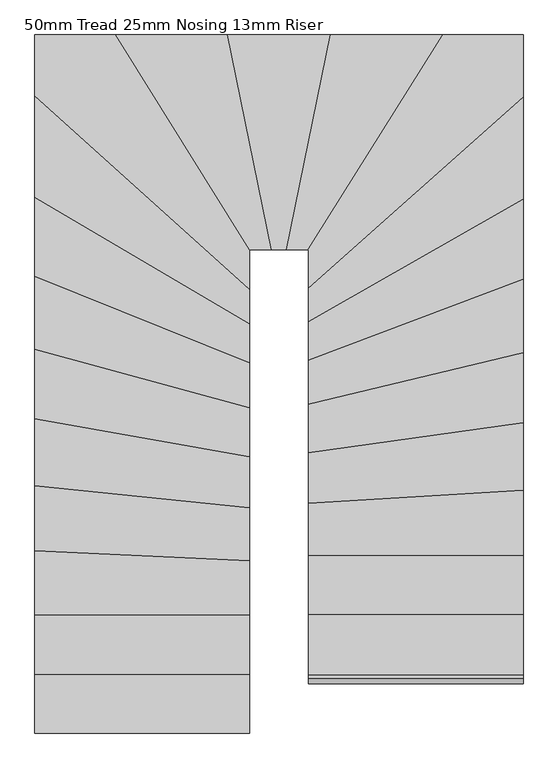
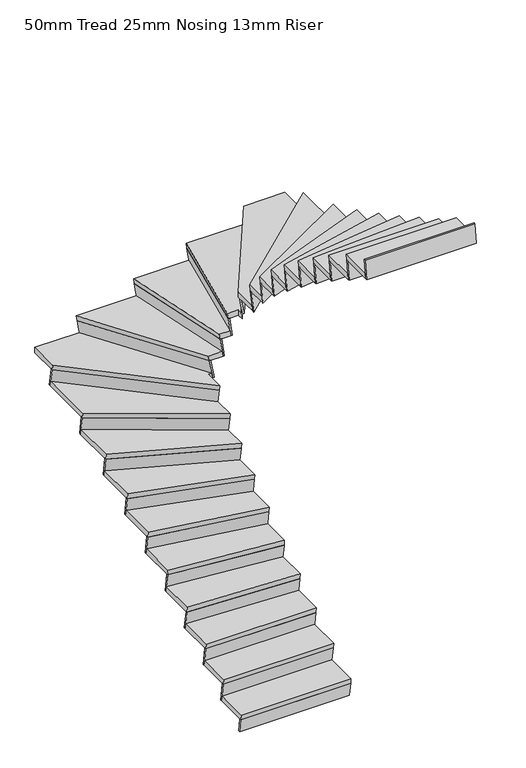
"""IFC4 building model written with IfcOpenShell, lengths in millimetres: stair flight geometry, 50mm Tread 25mm Nosing 13mm Riser."""

from ifc_helpers import new_model, si_unit, origin, place, context, project, spatial, faceted_brep, source, transform, mapped, element, save


def stair_flight_50mm_tread_25mm_nosing_13mm_riser_90fcb94b(model_context):
    return source(origin(), model_context, "Body", "Brep", [
        faceted_brep([(-7658.1394344, -389.3306191, 173.9130435), (-7658.1394344, -382.1431191, 123.9130435), (-8658.1652156, -382.1431191, 123.9130435), (-8658.1652156, -389.3306191, 173.9130435), (-8658.1652156, -689.3306191, 173.9130435), (-7658.1394344, -689.3306191, 173.9130435), (-7658.1394344, -682.1431191, 123.9130435), (-8658.1652156, -682.1431191, 123.9130435)], [[[0, 1, 2, 3]], [[3, 4, 5, 0]], [[2, 1, 6, 7]], [[4, 3, 2, 7]], [[0, 5, 6, 1]], [[5, 4, 7, 6]]]),
        faceted_brep([(-7658.1394344, -682.1431191, 123.9130435), (-7658.1394344, -664.3306191, 0.0), (-7658.1394344, -651.7021291, 0.0), (-7658.1394344, -669.5146291, 123.9130435), (-8658.1652156, -682.1431191, 123.9130435), (-8658.1652156, -669.5146291, 123.9130435), (-8658.1652156, -651.7021291, 0.0), (-8658.1652156, -664.3306191, 0.0)], [[[0, 1, 2, 3]], [[4, 5, 6, 7]], [[1, 0, 4, 7]], [[2, 1, 7, 6]], [[3, 2, 6, 5]], [[0, 3, 5, 4]]]),
        faceted_brep([(-7658.1394344, -407.1431191, 297.826087), (-7658.1394344, -382.1431191, 123.9130435), (-7658.1394344, -369.5146291, 123.9130435), (-7658.1394344, -394.5146291, 297.826087), (-8658.1652156, -407.1431191, 297.826087), (-8658.1652156, -394.5146291, 297.826087), (-8658.1652156, -369.5146291, 123.9130435), (-8658.1652156, -382.1431191, 123.9130435)], [[[0, 1, 2, 3]], [[4, 5, 6, 7]], [[1, 0, 4, 7]], [[2, 1, 7, 6]], [[3, 2, 6, 5]], [[0, 3, 5, 4]]]),
        faceted_brep([(-8658.1652156, -114.3306191, 347.826087), (-8658.1652156, -414.3306191, 347.826087), (-7658.1394344, -414.3306191, 347.826087), (-7658.1394344, -114.3306191, 347.826087), (-8658.1652156, -107.1431191, 297.826087), (-7658.1394344, -107.1431191, 297.826087), (-7658.1394344, -407.1431191, 297.826087), (-8658.1652156, -407.1431191, 297.826087)], [[[0, 1, 2, 3]], [[4, 5, 6, 7]], [[1, 0, 4, 7]], [[3, 2, 6, 5]], [[3, 5, 4, 0]], [[2, 1, 7, 6]]]),
        faceted_brep([(-7658.1394344, -132.1431191, 471.7391304), (-7658.1394344, -107.1431191, 297.826087), (-7658.1394344, -94.5146291, 297.826087), (-7658.1394344, -119.5146291, 471.7391304), (-8658.1652156, -132.1431191, 471.7391304), (-8658.1652156, -119.5146291, 471.7391304), (-8658.1652156, -94.5146291, 297.826087), (-8658.1652156, -107.1431191, 297.826087)], [[[0, 1, 2, 3]], [[4, 5, 6, 7]], [[1, 0, 4, 7]], [[2, 1, 7, 6]], [[3, 2, 6, 5]], [[0, 3, 5, 4]]]),
        faceted_brep([(-8658.1652156, 184.0364565, 521.7391304), (-8658.1652156, -139.3306191, 521.7391304), (-7658.1394344, -139.3306191, 521.7391304), (-7658.1394344, 137.3567478, 521.7391304), (-8658.1652156, 191.2317826, 471.7391304), (-7658.1394344, 144.5520739, 471.7391304), (-7658.1394344, -132.1431191, 471.7391304), (-8658.1652156, -132.1431191, 471.7391304)], [[[0, 1, 2, 3]], [[4, 5, 6, 7]], [[1, 0, 4, 7]], [[3, 2, 6, 5]], [[3, 5, 4, 0]], [[2, 1, 7, 6]]]),
        faceted_brep([(-7658.1394344, 119.5248527, 645.6521739), (-7658.1394344, 144.5520739, 471.7391304), (-7658.1394344, 157.1943144, 471.7391304), (-7658.1394344, 132.1670932, 645.6521739), (-8658.1652156, 166.2045614, 645.6521739), (-8658.1652156, 178.8468019, 645.6521739), (-8658.1652156, 203.8740231, 471.7391304), (-8658.1652156, 191.2317826, 471.7391304)], [[[0, 1, 2, 3]], [[4, 5, 6, 7]], [[1, 0, 4, 7]], [[2, 1, 7, 6]], [[3, 2, 6, 5]], [[0, 3, 5, 4]]]),
        faceted_brep([(-8658.1652156, 487.9562155, 695.6521739), (-8658.1652156, 159.0092353, 695.6521739), (-7658.1394344, 112.3295266, 695.6521739), (-7658.1394344, 383.6537717, 695.6521739), (-8658.1652156, 495.1827041, 645.6521739), (-7658.1394344, 390.8802603, 645.6521739), (-7658.1394344, 119.5248527, 645.6521739), (-8658.1652156, 166.2045614, 645.6521739)], [[[0, 1, 2, 3]], [[4, 5, 6, 7]], [[1, 0, 4, 7]], [[3, 2, 6, 5]], [[3, 5, 4, 0]], [[2, 1, 7, 6]]]),
        faceted_brep([(-7658.1394344, 365.7446477, 819.5652174), (-7658.1394344, 390.8802603, 645.6521739), (-7658.1394344, 403.5772537, 645.6521739), (-7658.1394344, 378.441641, 819.5652174), (-8658.1652156, 470.0470915, 819.5652174), (-8658.1652156, 482.7440848, 819.5652174), (-8658.1652156, 507.8796975, 645.6521739), (-8658.1652156, 495.1827041, 645.6521739)], [[[0, 1, 2, 3]], [[4, 5, 6, 7]], [[1, 0, 4, 7]], [[2, 1, 7, 6]], [[3, 2, 6, 5]], [[0, 3, 5, 4]]]),
        faceted_brep([(-8658.1652156, 799.6725249, 869.5652174), (-8658.1652156, 462.8206028, 869.5652174), (-7658.1394344, 358.518159, 869.5652174), (-7658.1394344, 622.4453627, 869.5652174), (-8658.1652156, 806.9720243, 819.5652174), (-7658.1394344, 629.7448621, 819.5652174), (-7658.1394344, 365.7446477, 819.5652174), (-8658.1652156, 470.0470915, 819.5652174)], [[[0, 1, 2, 3]], [[4, 5, 6, 7]], [[1, 0, 4, 7]], [[3, 2, 6, 5]], [[3, 5, 4, 0]], [[2, 1, 7, 6]]]),
        faceted_brep([(-7658.1394344, 604.3552992, 993.4782609), (-7658.1394344, 629.7448621, 819.5652174), (-7658.1394344, 642.5701357, 819.5652174), (-7658.1394344, 617.1805728, 993.4782609), (-8658.1652156, 781.5824614, 993.4782609), (-8658.1652156, 794.407735, 993.4782609), (-8658.1652156, 819.7972979, 819.5652174), (-8658.1652156, 806.9720243, 819.5652174)], [[[0, 1, 2, 3]], [[4, 5, 6, 7]], [[1, 0, 4, 7]], [[2, 1, 7, 6]], [[3, 2, 6, 5]], [[0, 3, 5, 4]]]),
        faceted_brep([(-8658.1652156, 1122.8219805, 1043.4782609), (-8658.1652156, 774.282962, 1043.4782609), (-7658.1394344, 597.0557998, 1043.4782609), (-7658.1394344, 850.3396239, 1043.4782609), (-8658.1652156, 1130.2715142, 993.4782609), (-7658.1394344, 857.7891576, 993.4782609), (-7658.1394344, 604.3552992, 993.4782609), (-8658.1652156, 781.5824614, 993.4782609)], [[[0, 1, 2, 3]], [[4, 5, 6, 7]], [[1, 0, 4, 7]], [[3, 2, 6, 5]], [[3, 5, 4, 0]], [[2, 1, 7, 6]]]),
        faceted_brep([(-7658.1394344, 831.8777363, 1167.3913043), (-7658.1394344, 857.7891576, 993.4782609), (-7658.1394344, 870.8780426, 993.4782609), (-7658.1394344, 844.9666213, 1167.3913043), (-8658.1652156, 1104.3600929, 1167.3913043), (-8658.1652156, 1117.4489779, 1167.3913043), (-8658.1652156, 1143.3603992, 993.4782609), (-8658.1652156, 1130.2715142, 993.4782609)], [[[0, 1, 2, 3]], [[4, 5, 6, 7]], [[1, 0, 4, 7]], [[2, 1, 7, 6]], [[3, 2, 6, 5]], [[0, 3, 5, 4]]]),
        faceted_brep([(-8658.1652156, 1463.7049519, 1217.3913043), (-8658.1652156, 1096.9105592, 1217.3913043), (-7658.1394344, 824.4282026, 1217.3913043), (-7658.1394344, 1061.5258249, 1217.3913043), (-8658.1652156, 1471.4519291, 1167.3913043), (-7658.1394344, 1069.2728021, 1167.3913043), (-7658.1394344, 831.8777363, 1167.3913043), (-8658.1652156, 1104.3600929, 1167.3913043)], [[[0, 1, 2, 3]], [[4, 5, 6, 7]], [[1, 0, 4, 7]], [[3, 2, 6, 5]], [[3, 5, 4, 0]], [[2, 1, 7, 6]]]),
        faceted_brep([(-7658.1394344, 1042.3267946, 1341.3043478), (-7658.1394344, 1069.2728021, 1167.3913043), (-7658.1394344, 1082.8842975, 1167.3913043), (-7658.1394344, 1055.93829, 1341.3043478), (-8658.1652156, 1444.5059216, 1341.3043478), (-8658.1652156, 1458.117417, 1341.3043478), (-8658.1652156, 1485.0634245, 1167.3913043), (-8658.1652156, 1471.4519291, 1167.3913043)], [[[0, 1, 2, 3]], [[4, 5, 6, 7]], [[1, 0, 4, 7]], [[2, 1, 7, 6]], [[3, 2, 6, 5]], [[0, 3, 5, 4]]]),
        faceted_brep([(-8658.1652156, 1834.2446243, 1391.3043478), (-8658.1652156, 1436.7589444, 1391.3043478), (-7658.1394344, 1034.5798174, 1391.3043478), (-7658.1394344, 1245.1252445, 1391.3043478), (-8658.1652156, 1842.5865959, 1341.3043478), (-7658.1394344, 1253.4672161, 1341.3043478), (-7658.1394344, 1042.3267946, 1341.3043478), (-8658.1652156, 1444.5059216, 1341.3043478)], [[[0, 1, 2, 3]], [[4, 5, 6, 7]], [[1, 0, 4, 7]], [[3, 2, 6, 5]], [[3, 5, 4, 0]], [[2, 1, 7, 6]]]),
        faceted_brep([(-7658.1394344, 1224.4516627, 1515.2173913), (-7658.1394344, 1253.4672161, 1341.3043478), (-7658.1394344, 1268.1241212, 1341.3043478), (-7658.1394344, 1239.1085677, 1515.2173913), (-8658.1652156, 1813.5710424, 1515.2173913), (-8658.1652156, 1828.2279475, 1515.2173913), (-8658.1652156, 1857.243501, 1341.3043478), (-8658.1652156, 1842.5865959, 1341.3043478)], [[[0, 1, 2, 3]], [[4, 5, 6, 7]], [[1, 0, 4, 7]], [[2, 1, 7, 6]], [[3, 2, 6, 5]], [[0, 3, 5, 4]]]),
        faceted_brep([(-8658.1652156, 2311.0566713, 1565.2173913), (-8658.1652156, 1805.2290708, 1565.2173913), (-7658.1394344, 1216.109691, 1565.2173913), (-7658.1394344, 1410.1980697, 1565.2173913), (-8658.1652156, 2320.7304813, 1515.2173913), (-7658.1394344, 1419.8718797, 1515.2173913), (-7658.1394344, 1224.4516627, 1515.2173913), (-8658.1652156, 1813.5710424, 1515.2173913)], [[[0, 1, 2, 3]], [[4, 5, 6, 7]], [[1, 0, 4, 7]], [[3, 2, 6, 5]], [[3, 5, 4, 0]], [[2, 1, 7, 6]]]),
        faceted_brep([(-7658.1394344, 1386.223845, 1689.1304348), (-7658.1394344, 1419.8718797, 1515.2173913), (-7658.1394344, 1436.8688344, 1515.2173913), (-7658.1394344, 1403.2207998, 1689.1304348), (-8658.1652156, 2287.0824466, 1689.1304348), (-8658.1652156, 2304.0794014, 1689.1304348), (-8658.1652156, 2337.727436, 1515.2173913), (-8658.1652156, 2320.7304813, 1515.2173913)], [[[0, 1, 2, 3]], [[4, 5, 6, 7]], [[1, 0, 4, 7]], [[2, 1, 7, 6]], [[3, 2, 6, 5]], [[0, 3, 5, 4]]]),
        faceted_brep([(-8253.2071853, 2560.492595, 1739.1304348), (-8658.1652156, 2560.492595, 1739.1304348), (-8658.1652156, 2277.4086367, 1739.1304348), (-7658.1394344, 1376.5500351, 1739.1304348), (-7658.1394344, 1560.4668138, 1739.1304348), (-7627.5175626, 1560.4668138, 1739.1304348), (-8244.7287763, 2560.492595, 1689.1304348), (-7619.0391536, 1560.4668138, 1689.1304348), (-7658.1394344, 1560.4668138, 1689.1304348), (-7658.1394344, 1386.223845, 1689.1304348), (-8658.1652156, 2287.0824466, 1689.1304348), (-8658.1652156, 2560.492595, 1689.1304348)], [[[0, 1, 2, 3, 4, 5]], [[6, 7, 8, 9, 10, 11]], [[1, 0, 6, 11]], [[2, 1, 11, 10]], [[4, 3, 9, 8]], [[5, 4, 8, 7]], [[5, 7, 6, 0]], [[3, 2, 10, 9]]]),
        faceted_brep([(-7648.5292718, 1560.4668138, 1863.0434783), (-7619.0391536, 1560.4668138, 1689.1304348), (-7604.142527, 1560.4668138, 1689.1304348), (-7633.6326453, 1560.4668138, 1863.0434783), (-8274.2188945, 2560.492595, 1863.0434783), (-8259.322268, 2560.492595, 1863.0434783), (-8229.8321498, 2560.492595, 1689.1304348), (-8244.7287763, 2560.492595, 1689.1304348)], [[[0, 1, 2, 3]], [[4, 5, 6, 7]], [[1, 0, 4, 7]], [[2, 1, 7, 6]], [[3, 2, 6, 5]], [[0, 3, 5, 4]]]),
        faceted_brep([(-7734.1295481, 2560.492595, 1913.0434783), (-8282.6973035, 2560.492595, 1913.0434783), (-7657.0076808, 1560.4668138, 1913.0434783), (-7531.1295481, 1560.4668138, 1913.0434783), (-7726.7954558, 2560.492595, 1863.0434783), (-7523.7954558, 1560.4668138, 1863.0434783), (-7648.5292718, 1560.4668138, 1863.0434783), (-8274.2188945, 2560.492595, 1863.0434783)], [[[0, 1, 2, 3]], [[4, 5, 6, 7]], [[1, 0, 4, 7]], [[3, 2, 6, 5]], [[3, 5, 4, 0]], [[2, 1, 7, 6]]]),
        faceted_brep([(-7549.3053421, 1560.4668138, 2036.9565217), (-7523.7954558, 1560.4668138, 1863.0434783), (-7510.9094021, 1560.4668138, 1863.0434783), (-7536.4192883, 1560.4668138, 2036.9565217), (-7752.3053421, 2560.492595, 2036.9565217), (-7739.4192883, 2560.492595, 2036.9565217), (-7713.9094021, 2560.492595, 1863.0434783), (-7726.7954558, 2560.492595, 1863.0434783)], [[[0, 1, 2, 3]], [[4, 5, 6, 7]], [[1, 0, 4, 7]], [[2, 1, 7, 6]], [[3, 2, 6, 5]], [[0, 3, 5, 4]]]),
        faceted_brep([(-7256.1295481, 2560.492595, 2086.9565217), (-7759.6394344, 2560.492595, 2086.9565217), (-7556.6394344, 1560.4668138, 2086.9565217), (-7459.1295481, 1560.4668138, 2086.9565217), (-7248.7954558, 2560.492595, 2036.9565217), (-7451.7954558, 1560.4668138, 2036.9565217), (-7549.3053421, 1560.4668138, 2036.9565217), (-7752.3053421, 2560.492595, 2036.9565217)], [[[0, 1, 2, 3]], [[4, 5, 6, 7]], [[1, 0, 4, 7]], [[3, 2, 6, 5]], [[3, 5, 4, 0]], [[2, 1, 7, 6]]]),
        faceted_brep([(-7477.3053421, 1560.4668138, 2210.8695652), (-7451.7954558, 1560.4668138, 2036.9565217), (-7438.9094021, 1560.4668138, 2036.9565217), (-7464.4192883, 1560.4668138, 2210.8695652), (-7274.3053421, 2560.492595, 2210.8695652), (-7261.4192883, 2560.492595, 2210.8695652), (-7235.9094021, 2560.492595, 2036.9565217), (-7248.7954558, 2560.492595, 2036.9565217)], [[[0, 1, 2, 3]], [[4, 5, 6, 7]], [[1, 0, 4, 7]], [[2, 1, 7, 6]], [[3, 2, 6, 5]], [[0, 3, 5, 4]]]),
        faceted_brep([(-6727.6298091, 2560.492595, 2260.8695652), (-7281.6394344, 2560.492595, 2260.8695652), (-7484.6394344, 1560.4668138, 2260.8695652), (-7383.1394344, 1560.4668138, 2260.8695652), (-7383.1394344, 1516.945701, 2260.8695652), (-6719.1419248, 2560.492595, 2210.8695652), (-7383.1394344, 1503.4333055, 2210.8695652), (-7383.1394344, 1560.4668138, 2210.8695652), (-7477.3053421, 1560.4668138, 2210.8695652), (-7274.3053421, 2560.492595, 2210.8695652)], [[[0, 1, 2, 3, 4]], [[5, 6, 7, 8, 9]], [[1, 0, 5, 9]], [[3, 2, 8, 7]], [[4, 3, 7, 6]], [[4, 6, 5, 0]], [[2, 1, 9, 8]]]),
        faceted_brep([(-7376.8366036, 1560.4668138, 2384.7826087), (-7347.3135277, 1560.4668138, 2210.8695652), (-7332.4002529, 1560.4668138, 2210.8695652), (-7361.9233288, 1560.4668138, 2384.7826087), (-6748.6650007, 2560.492595, 2384.7826087), (-6733.7517259, 2560.492595, 2384.7826087), (-6704.22865, 2560.492595, 2210.8695652), (-6719.1419248, 2560.492595, 2210.8695652)], [[[0, 1, 2, 3]], [[4, 5, 6, 7]], [[1, 0, 4, 7]], [[2, 1, 7, 6]], [[3, 2, 6, 5]], [[0, 3, 5, 4]]]),
        faceted_brep([(-6383.1136531, 2236.961945, 2434.7826087), (-6383.1136531, 2560.492595, 2434.7826087), (-6757.152885, 2560.492595, 2434.7826087), (-7385.3244879, 1560.4668138, 2434.7826087), (-7383.1394344, 1560.4668138, 2434.7826087), (-7383.1394344, 1348.82239, 2434.7826087), (-6383.1136531, 2227.3490804, 2384.7826087), (-7383.1394344, 1339.2095254, 2384.7826087), (-7383.1394344, 1560.4668138, 2384.7826087), (-7376.8366036, 1560.4668138, 2384.7826087), (-6748.6650007, 2560.492595, 2384.7826087), (-6383.1136531, 2560.492595, 2384.7826087), (-7383.1394344, 1560.4668138, 2421.9110056)], [[[0, 1, 2, 3, 4, 5]], [[6, 7, 8, 9, 10, 11]], [[1, 0, 6, 11]], [[2, 1, 11, 10]], [[4, 3, 12]], [[5, 4, 12, 8, 7]], [[5, 7, 6, 0]], [[12, 9, 8]], [[9, 12, 3, 2, 10]]]),
        faceted_brep([(-7383.1394344, 1372.6455763, 2558.6956522), (-7383.1394344, 1339.2095254, 2384.7826087), (-7383.1394344, 1322.319652, 2384.7826087), (-7383.1394344, 1355.7557029, 2558.6956522), (-6383.1136531, 2260.7851313, 2558.6956522), (-6383.1136531, 2243.8952579, 2558.6956522), (-6383.1136531, 2210.459207, 2384.7826087), (-6383.1136531, 2227.3490804, 2384.7826087)], [[[0, 1, 2, 3]], [[4, 5, 6, 7]], [[1, 0, 4, 7]], [[2, 1, 7, 6]], [[3, 2, 6, 5]], [[0, 3, 5, 4]]]),
        faceted_brep([(-6383.1136531, 1767.1523947, 2608.6956522), (-6383.1136531, 2270.3979959, 2608.6956522), (-7383.1394344, 1382.2584409, 2608.6956522), (-7383.1394344, 1196.62143, 2608.6956522), (-6383.1136531, 1758.8774349, 2558.6956522), (-7383.1394344, 1188.3464703, 2558.6956522), (-7383.1394344, 1372.6455763, 2558.6956522), (-6383.1136531, 2260.7851313, 2558.6956522)], [[[0, 1, 2, 3]], [[4, 5, 6, 7]], [[1, 0, 4, 7]], [[3, 2, 6, 5]], [[3, 5, 4, 0]], [[2, 1, 7, 6]]]),
        faceted_brep([(-7383.1394344, 1217.1289389, 2732.6086957), (-7383.1394344, 1188.3464703, 2558.6956522), (-7383.1394344, 1173.8073056, 2558.6956522), (-7383.1394344, 1202.5897742, 2732.6086957), (-6383.1136531, 1787.6599035, 2732.6086957), (-6383.1136531, 1773.1207389, 2732.6086957), (-6383.1136531, 1744.3382702, 2558.6956522), (-6383.1136531, 1758.8774349, 2558.6956522)], [[[0, 1, 2, 3]], [[4, 5, 6, 7]], [[1, 0, 4, 7]], [[2, 1, 7, 6]], [[3, 2, 6, 5]], [[0, 3, 5, 4]]]),
        faceted_brep([(-6383.1136531, 1397.5341685, 2782.6086957), (-6383.1136531, 1795.9348633, 2782.6086957), (-7383.1394344, 1225.4038986, 2782.6086957), (-7383.1394344, 1020.3665908, 2782.6086957), (-6383.1136531, 1389.8524556, 2732.6086957), (-7383.1394344, 1012.6848779, 2732.6086957), (-7383.1394344, 1217.1289389, 2732.6086957), (-6383.1136531, 1787.6599035, 2732.6086957)], [[[0, 1, 2, 3]], [[4, 5, 6, 7]], [[1, 0, 4, 7]], [[3, 2, 6, 5]], [[3, 5, 4, 0]], [[2, 1, 7, 6]]]),
        faceted_brep([(-7383.1394344, 1039.4038792, 2906.5217391), (-7383.1394344, 1012.6848779, 2732.6086957), (-7383.1394344, 999.1880523, 2732.6086957), (-7383.1394344, 1025.9070536, 2906.5217391), (-6383.1136531, 1416.5714569, 2906.5217391), (-6383.1136531, 1403.0746313, 2906.5217391), (-6383.1136531, 1376.35563, 2732.6086957), (-6383.1136531, 1389.8524556, 2732.6086957)], [[[0, 1, 2, 3]], [[4, 5, 6, 7]], [[1, 0, 4, 7]], [[2, 1, 7, 6]], [[3, 2, 6, 5]], [[0, 3, 5, 4]]]),
        faceted_brep([(-6383.1136531, 1055.4648272, 2956.5217391), (-6383.1136531, 1424.2531698, 2956.5217391), (-7383.1394344, 1047.0855921, 2956.5217391), (-7383.1394344, 814.4422104, 2956.5217391), (-6383.1136531, 1048.0715168, 2906.5217391), (-7383.1394344, 807.0489, 2906.5217391), (-7383.1394344, 1039.4038792, 2906.5217391), (-6383.1136531, 1416.5714569, 2906.5217391)], [[[0, 1, 2, 3]], [[4, 5, 6, 7]], [[1, 0, 4, 7]], [[3, 2, 6, 5]], [[3, 5, 4, 0]], [[2, 1, 7, 6]]]),
        faceted_brep([(-7383.1394344, 832.7647621, 3080.4347826), (-7383.1394344, 807.0489, 2906.5217391), (-7383.1394344, 794.0587997, 2906.5217391), (-7383.1394344, 819.7746618, 3080.4347826), (-6383.1136531, 1073.787379, 3080.4347826), (-6383.1136531, 1060.7972786, 3080.4347826), (-6383.1136531, 1035.0814165, 2906.5217391), (-6383.1136531, 1048.0715168, 2906.5217391)], [[[0, 1, 2, 3]], [[4, 5, 6, 7]], [[1, 0, 4, 7]], [[2, 1, 7, 6]], [[3, 2, 6, 5]], [[0, 3, 5, 4]]]),
        faceted_brep([(-6383.1136531, 730.4117187, 3130.4347826), (-6383.1136531, 1081.1806893, 3130.4347826), (-7383.1394344, 840.1580725, 3130.4347826), (-7383.1394344, 590.4396395, 3130.4347826), (-6383.1136531, 723.1541544, 3080.4347826), (-7383.1394344, 583.1820752, 3080.4347826), (-7383.1394344, 832.7647621, 3080.4347826), (-6383.1136531, 1073.787379, 3080.4347826)], [[[0, 1, 2, 3]], [[4, 5, 6, 7]], [[1, 0, 4, 7]], [[3, 2, 6, 5]], [[3, 5, 4, 0]], [[2, 1, 7, 6]]]),
        faceted_brep([(-7383.1394344, 608.425777, 3254.3478261), (-7383.1394344, 583.1820752, 3080.4347826), (-7383.1394344, 570.4304817, 3080.4347826), (-7383.1394344, 595.6741836, 3254.3478261), (-6383.1136531, 748.3978563, 3254.3478261), (-6383.1136531, 735.6462628, 3254.3478261), (-6383.1136531, 710.402561, 3080.4347826), (-6383.1136531, 723.1541544, 3080.4347826)], [[[0, 1, 2, 3]], [[4, 5, 6, 7]], [[1, 0, 4, 7]], [[2, 1, 7, 6]], [[3, 2, 6, 5]], [[0, 3, 5, 4]]]),
        faceted_brep([(-6383.1136531, 416.6192128, 3304.3478261), (-6383.1136531, 755.6554205, 3304.3478261), (-7383.1394344, 615.6833413, 3304.3478261), (-7383.1394344, 354.6235596, 3304.3478261), (-6383.1136531, 409.4179143, 3254.3478261), (-7383.1394344, 347.4222611, 3254.3478261), (-7383.1394344, 608.425777, 3254.3478261), (-6383.1136531, 748.3978563, 3254.3478261)], [[[0, 1, 2, 3]], [[4, 5, 6, 7]], [[1, 0, 4, 7]], [[3, 2, 6, 5]], [[3, 5, 4, 0]], [[2, 1, 7, 6]]]),
        faceted_brep([(-7383.1394344, 372.4702559, 3428.2608696), (-7383.1394344, 347.4222611, 3254.3478261), (-7383.1394344, 334.7695271, 3254.3478261), (-7383.1394344, 359.8175218, 3428.2608696), (-6383.1136531, 434.465909, 3428.2608696), (-6383.1136531, 421.813175, 3428.2608696), (-6383.1136531, 396.7651803, 3254.3478261), (-6383.1136531, 409.4179143, 3254.3478261)], [[[0, 1, 2, 3]], [[4, 5, 6, 7]], [[1, 0, 4, 7]], [[2, 1, 7, 6]], [[3, 2, 6, 5]], [[0, 3, 5, 4]]]),
        faceted_brep([(-6383.1136531, 110.6693809, 3478.2608696), (-6383.1136531, 441.6672075, 3478.2608696), (-7383.1394344, 379.6715543, 3478.2608696), (-7383.1394344, 110.6693809, 3478.2608696), (-6383.1136531, 103.4818809, 3428.2608696), (-7383.1394344, 103.4818809, 3428.2608696), (-7383.1394344, 372.4702559, 3428.2608696), (-6383.1136531, 434.465909, 3428.2608696)], [[[0, 1, 2, 3]], [[4, 5, 6, 7]], [[1, 0, 4, 7]], [[3, 2, 6, 5]], [[3, 5, 4, 0]], [[2, 1, 7, 6]]]),
        faceted_brep([(-7383.1394344, 128.4818809, 3602.173913), (-7383.1394344, 103.4818809, 3428.2608696), (-7383.1394344, 90.8533909, 3428.2608696), (-7383.1394344, 115.8533909, 3602.173913), (-6383.1136531, 128.4818809, 3602.173913), (-6383.1136531, 115.8533909, 3602.173913), (-6383.1136531, 90.8533909, 3428.2608696), (-6383.1136531, 103.4818809, 3428.2608696)], [[[0, 1, 2, 3]], [[4, 5, 6, 7]], [[1, 0, 4, 7]], [[2, 1, 7, 6]], [[3, 2, 6, 5]], [[0, 3, 5, 4]]]),
        faceted_brep([(-6383.1136531, -164.3306191, 3652.173913), (-6383.1136531, 135.6693809, 3652.173913), (-7383.1394344, 135.6693809, 3652.173913), (-7383.1394344, -164.3306191, 3652.173913), (-6383.1136531, -171.5181191, 3602.173913), (-7383.1394344, -171.5181191, 3602.173913), (-7383.1394344, 128.4818809, 3602.173913), (-6383.1136531, 128.4818809, 3602.173913)], [[[0, 1, 2, 3]], [[4, 5, 6, 7]], [[1, 0, 4, 7]], [[3, 2, 6, 5]], [[3, 5, 4, 0]], [[2, 1, 7, 6]]]),
        faceted_brep([(-7383.1394344, -146.5181191, 3776.0869565), (-7383.1394344, -171.5181191, 3602.173913), (-7383.1394344, -184.1466091, 3602.173913), (-7383.1394344, -159.1466091, 3776.0869565), (-6383.1136531, -146.5181191, 3776.0869565), (-6383.1136531, -159.1466091, 3776.0869565), (-6383.1136531, -184.1466091, 3602.173913), (-6383.1136531, -171.5181191, 3602.173913)], [[[0, 1, 2, 3]], [[4, 5, 6, 7]], [[1, 0, 4, 7]], [[2, 1, 7, 6]], [[3, 2, 6, 5]], [[0, 3, 5, 4]]]),
        faceted_brep([(-7383.1394344, -421.5181191, 3950.0), (-7383.1394344, -446.5181191, 3776.0869565), (-7383.1394344, -459.1466091, 3776.0869565), (-7383.1394344, -434.1466091, 3950.0), (-6383.1136531, -421.5181191, 3950.0), (-6383.1136531, -434.1466091, 3950.0), (-6383.1136531, -459.1466091, 3776.0869565), (-6383.1136531, -446.5181191, 3776.0869565)], [[[0, 1, 2, 3]], [[4, 5, 6, 7]], [[1, 0, 4, 7]], [[2, 1, 7, 6]], [[3, 2, 6, 5]], [[0, 3, 5, 4]]]),
        faceted_brep([(-6383.1136531, -439.3306191, 3826.0869565), (-6383.1136531, -139.3306191, 3826.0869565), (-7383.1394344, -139.3306191, 3826.0869565), (-7383.1394344, -439.3306191, 3826.0869565), (-6383.1136531, -446.5181191, 3776.0869565), (-7383.1394344, -446.5181191, 3776.0869565), (-7383.1394344, -146.5181191, 3776.0869565), (-6383.1136531, -146.5181191, 3776.0869565)], [[[0, 1, 2, 3]], [[4, 5, 6, 7]], [[1, 0, 4, 7]], [[3, 2, 6, 5]], [[3, 5, 4, 0]], [[2, 1, 7, 6]]]),
    ])


if __name__ == "__main__":
    model = new_model("IFC4")
    model_context = context("Model", 3, world=origin())
    ifc_project = project(units=[si_unit("LENGTHUNIT", "METRE", prefix="MILLI")], contexts=[model_context])
    site = spatial("IfcSite", under=ifc_project)
    building = spatial("IfcBuilding", under=site)
    placement = place(None, origin())
    stair_flight_50mm_tread_25mm_nosing_13mm_riser_shape = stair_flight_50mm_tread_25mm_nosing_13mm_riser_90fcb94b(model_context)
    element("IfcStairFlight", 1, ObjectType="50mm Tread 25mm Nosing 13mm Riser", at=placement, inside=building, context=model_context, shape_type="MappedRepresentation", body=[
        mapped(stair_flight_50mm_tread_25mm_nosing_13mm_riser_shape, transform((0.0, 0.0, 0.0), x_axis=(1.0, 0.0, 0.0), y_axis=(0.0, 1.0, 0.0), z_axis=(0.0, 0.0, 1.0))),
    ])
    save(model, "model.ifc")
